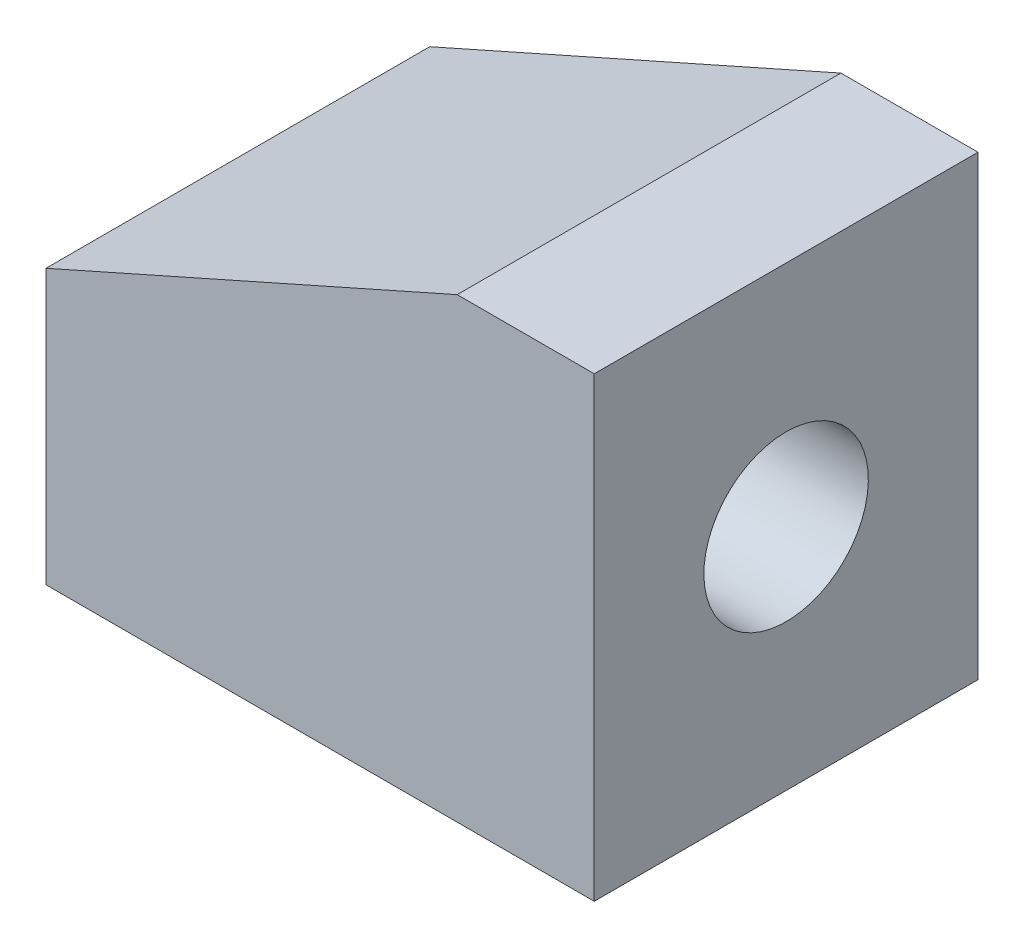
ISO-10303-21;
HEADER;
FILE_DESCRIPTION(('STEP AP214'),'2;1');
FILE_NAME('part.step','',(''),(''),'','','');
FILE_SCHEMA(('AUTOMOTIVE_DESIGN { 1 0 10303 214 1 1 1 1 }'));
ENDSEC;
DATA;
#1=APPLICATION_CONTEXT('core data for automotive mechanical design processes');
#2=APPLICATION_PROTOCOL_DEFINITION('international standard','automotive_design',2000,#1);
#3=PRODUCT_CONTEXT('',#1,'mechanical');
#4=PRODUCT('Part','Part','',(#3));
#5=PRODUCT_RELATED_PRODUCT_CATEGORY('part','',(#4));
#6=PRODUCT_DEFINITION_FORMATION('','',#4);
#7=PRODUCT_DEFINITION_CONTEXT('part definition',#1,'design');
#8=PRODUCT_DEFINITION('design','',#6,#7);
#9=PRODUCT_DEFINITION_SHAPE('','',#8);
#10=(LENGTH_UNIT() NAMED_UNIT(*) SI_UNIT(.MILLI.,.METRE.));
#11=(NAMED_UNIT(*) PLANE_ANGLE_UNIT() SI_UNIT($,.RADIAN.));
#12=(NAMED_UNIT(*) SI_UNIT($,.STERADIAN.) SOLID_ANGLE_UNIT());
#13=UNCERTAINTY_MEASURE_WITH_UNIT(LENGTH_MEASURE(1.E-05),#10,'distance_accuracy_value','');
#14=(GEOMETRIC_REPRESENTATION_CONTEXT(3) GLOBAL_UNCERTAINTY_ASSIGNED_CONTEXT((#13)) GLOBAL_UNIT_ASSIGNED_CONTEXT((#10,
#11,#12)) REPRESENTATION_CONTEXT('',''));
#15=CARTESIAN_POINT('',(0.,0.,0.));
#16=DIRECTION('',(0.,0.,1.));
#17=DIRECTION('',(1.,0.,0.));
#18=AXIS2_PLACEMENT_3D('',#15,#16,#17);
#19=CARTESIAN_POINT('',(-30.,0.,21.));
#20=DIRECTION('',(1.,0.,0.));
#21=DIRECTION('',(0.,0.,-1.));
#22=AXIS2_PLACEMENT_3D('',#19,#20,#21);
#23=PLANE('',#22);
#24=DIRECTION('',(0.,-1.,0.));
#25=VECTOR('',#24,1.);
#26=CARTESIAN_POINT('',(-30.,0.,-21.));
#27=LINE('',#26,#25);
#28=CARTESIAN_POINT('',(-30.,30.,-21.));
#29=VERTEX_POINT('',#28);
#30=CARTESIAN_POINT('',(-30.,0.,-21.));
#31=VERTEX_POINT('',#30);
#32=EDGE_CURVE('E117',#29,#31,#27,.T.);
#33=ORIENTED_EDGE('',*,*,#32,.T.);
#34=DIRECTION('',(0.,0.,-1.));
#35=VECTOR('',#34,1.);
#36=CARTESIAN_POINT('',(-30.,0.,21.));
#37=LINE('',#36,#35);
#38=CARTESIAN_POINT('',(-30.,0.,21.));
#39=VERTEX_POINT('',#38);
#40=EDGE_CURVE('E11',#39,#31,#37,.T.);
#41=ORIENTED_EDGE('',*,*,#40,.F.);
#42=DIRECTION('',(0.,-1.,0.));
#43=VECTOR('',#42,1.);
#44=CARTESIAN_POINT('',(-30.,0.,21.));
#45=LINE('',#44,#43);
#46=CARTESIAN_POINT('',(-30.,30.,21.));
#47=VERTEX_POINT('',#46);
#48=EDGE_CURVE('E127',#47,#39,#45,.T.);
#49=ORIENTED_EDGE('',*,*,#48,.F.);
#50=DIRECTION('',(0.,0.,-1.));
#51=VECTOR('',#50,1.);
#52=CARTESIAN_POINT('',(-30.,30.,21.));
#53=LINE('',#52,#51);
#54=EDGE_CURVE('E114',#47,#29,#53,.T.);
#55=ORIENTED_EDGE('',*,*,#54,.T.);
#56=EDGE_LOOP('',(#33,#41,#49,#55));
#57=FACE_BOUND('',#56,.T.);
#58=ADVANCED_FACE('F43',(#57),#23,.F.);
#59=CARTESIAN_POINT('',(30.,0.,21.));
#60=DIRECTION('',(0.,1.,0.));
#61=DIRECTION('',(0.,0.,1.));
#62=AXIS2_PLACEMENT_3D('',#59,#60,#61);
#63=PLANE('',#62);
#64=DIRECTION('',(1.,0.,0.));
#65=VECTOR('',#64,1.);
#66=CARTESIAN_POINT('',(30.,0.,-21.));
#67=LINE('',#66,#65);
#68=CARTESIAN_POINT('',(30.,0.,-21.));
#69=VERTEX_POINT('',#68);
#70=EDGE_CURVE('E120',#31,#69,#67,.T.);
#71=ORIENTED_EDGE('',*,*,#70,.T.);
#72=DIRECTION('',(0.,0.,-1.));
#73=VECTOR('',#72,1.);
#74=CARTESIAN_POINT('',(30.,0.,21.));
#75=LINE('',#74,#73);
#76=CARTESIAN_POINT('',(30.,0.,21.));
#77=VERTEX_POINT('',#76);
#78=EDGE_CURVE('E51',#77,#69,#75,.T.);
#79=ORIENTED_EDGE('',*,*,#78,.F.);
#80=DIRECTION('',(1.,0.,0.));
#81=VECTOR('',#80,1.);
#82=CARTESIAN_POINT('',(30.,0.,21.));
#83=LINE('',#82,#81);
#84=EDGE_CURVE('E91',#39,#77,#83,.T.);
#85=ORIENTED_EDGE('',*,*,#84,.F.);
#86=ORIENTED_EDGE('',*,*,#40,.T.);
#87=EDGE_LOOP('',(#71,#79,#85,#86));
#88=FACE_BOUND('',#87,.T.);
#89=ADVANCED_FACE('F144',(#88),#63,.F.);
#90=CARTESIAN_POINT('',(30.,50.,21.));
#91=DIRECTION('',(-1.,0.,0.));
#92=DIRECTION('',(0.,-1.,0.));
#93=AXIS2_PLACEMENT_3D('',#90,#91,#92);
#94=PLANE('',#93);
#95=CARTESIAN_POINT('',(30.,25.,0.));
#96=DIRECTION('',(1.,0.,0.));
#97=DIRECTION('',(0.,1.,0.));
#98=AXIS2_PLACEMENT_3D('',#95,#96,#97);
#99=CIRCLE('',#98,9.);
#100=CARTESIAN_POINT('',(30.,34.,0.));
#101=VERTEX_POINT('',#100);
#102=EDGE_CURVE('E159',#101,#101,#99,.T.);
#103=ORIENTED_EDGE('',*,*,#102,.F.);
#104=EDGE_LOOP('',(#103));
#105=FACE_BOUND('',#104,.T.);
#106=DIRECTION('',(0.,1.,0.));
#107=VECTOR('',#106,1.);
#108=CARTESIAN_POINT('',(30.,50.,-21.));
#109=LINE('',#108,#107);
#110=CARTESIAN_POINT('',(30.,50.,-21.));
#111=VERTEX_POINT('',#110);
#112=EDGE_CURVE('E107',#69,#111,#109,.T.);
#113=ORIENTED_EDGE('',*,*,#112,.T.);
#114=DIRECTION('',(0.,0.,-1.));
#115=VECTOR('',#114,1.);
#116=CARTESIAN_POINT('',(30.,50.,21.));
#117=LINE('',#116,#115);
#118=CARTESIAN_POINT('',(30.,50.,21.));
#119=VERTEX_POINT('',#118);
#120=EDGE_CURVE('E104',#119,#111,#117,.T.);
#121=ORIENTED_EDGE('',*,*,#120,.F.);
#122=DIRECTION('',(0.,1.,0.));
#123=VECTOR('',#122,1.);
#124=CARTESIAN_POINT('',(30.,50.,21.));
#125=LINE('',#124,#123);
#126=EDGE_CURVE('E100',#77,#119,#125,.T.);
#127=ORIENTED_EDGE('',*,*,#126,.F.);
#128=ORIENTED_EDGE('',*,*,#78,.T.);
#129=EDGE_LOOP('',(#113,#121,#127,#128));
#130=FACE_BOUND('',#129,.T.);
#131=ADVANCED_FACE('F106',(#105,#130),#94,.F.);
#132=CARTESIAN_POINT('',(15.,50.,21.));
#133=DIRECTION('',(0.,-1.,0.));
#134=DIRECTION('',(0.,0.,-1.));
#135=AXIS2_PLACEMENT_3D('',#132,#133,#134);
#136=PLANE('',#135);
#137=DIRECTION('',(-1.,0.,0.));
#138=VECTOR('',#137,1.);
#139=CARTESIAN_POINT('',(15.,50.,-21.));
#140=LINE('',#139,#138);
#141=CARTESIAN_POINT('',(15.,50.,-21.));
#142=VERTEX_POINT('',#141);
#143=EDGE_CURVE('E78',#111,#142,#140,.T.);
#144=ORIENTED_EDGE('',*,*,#143,.T.);
#145=DIRECTION('',(0.,0.,-1.));
#146=VECTOR('',#145,1.);
#147=CARTESIAN_POINT('',(15.,50.,21.));
#148=LINE('',#147,#146);
#149=CARTESIAN_POINT('',(15.,50.,21.));
#150=VERTEX_POINT('',#149);
#151=EDGE_CURVE('E108',#150,#142,#148,.T.);
#152=ORIENTED_EDGE('',*,*,#151,.F.);
#153=DIRECTION('',(-1.,0.,0.));
#154=VECTOR('',#153,1.);
#155=CARTESIAN_POINT('',(15.,50.,21.));
#156=LINE('',#155,#154);
#157=EDGE_CURVE('E101',#119,#150,#156,.T.);
#158=ORIENTED_EDGE('',*,*,#157,.F.);
#159=ORIENTED_EDGE('',*,*,#120,.T.);
#160=EDGE_LOOP('',(#144,#152,#158,#159));
#161=FACE_BOUND('',#160,.T.);
#162=ADVANCED_FACE('F112',(#161),#136,.F.);
#163=CARTESIAN_POINT('',(-30.,30.,21.));
#164=DIRECTION('',(0.406138466053448,-0.913811548620257,0.));
#165=DIRECTION('',(0.913811548620257,0.406138466053448,0.));
#166=AXIS2_PLACEMENT_3D('',#163,#164,#165);
#167=PLANE('',#166);
#168=DIRECTION('',(-0.913811548620257,-0.406138466053448,0.));
#169=VECTOR('',#168,1.);
#170=CARTESIAN_POINT('',(-30.,30.,-21.));
#171=LINE('',#170,#169);
#172=EDGE_CURVE('E84',#142,#29,#171,.T.);
#173=ORIENTED_EDGE('',*,*,#172,.T.);
#174=ORIENTED_EDGE('',*,*,#54,.F.);
#175=DIRECTION('',(-0.913811548620257,-0.406138466053448,0.));
#176=VECTOR('',#175,1.);
#177=CARTESIAN_POINT('',(-30.,30.,21.));
#178=LINE('',#177,#176);
#179=EDGE_CURVE('E56',#150,#47,#178,.T.);
#180=ORIENTED_EDGE('',*,*,#179,.F.);
#181=ORIENTED_EDGE('',*,*,#151,.T.);
#182=EDGE_LOOP('',(#173,#174,#180,#181));
#183=FACE_BOUND('',#182,.T.);
#184=ADVANCED_FACE('F133',(#183),#167,.F.);
#185=CARTESIAN_POINT('',(0.,0.,21.));
#186=DIRECTION('',(0.,0.,-1.));
#187=DIRECTION('',(-1.,0.,0.));
#188=AXIS2_PLACEMENT_3D('',#185,#186,#187);
#189=PLANE('',#188);
#190=ORIENTED_EDGE('',*,*,#48,.T.);
#191=ORIENTED_EDGE('',*,*,#84,.T.);
#192=ORIENTED_EDGE('',*,*,#126,.T.);
#193=ORIENTED_EDGE('',*,*,#157,.T.);
#194=ORIENTED_EDGE('',*,*,#179,.T.);
#195=EDGE_LOOP('',(#190,#191,#192,#193,#194));
#196=FACE_BOUND('',#195,.T.);
#197=ADVANCED_FACE('F97',(#196),#189,.F.);
#198=CARTESIAN_POINT('',(0.,0.,-21.));
#199=DIRECTION('',(0.,0.,-1.));
#200=DIRECTION('',(-1.,0.,0.));
#201=AXIS2_PLACEMENT_3D('',#198,#199,#200);
#202=PLANE('',#201);
#203=ORIENTED_EDGE('',*,*,#32,.F.);
#204=ORIENTED_EDGE('',*,*,#172,.F.);
#205=ORIENTED_EDGE('',*,*,#143,.F.);
#206=ORIENTED_EDGE('',*,*,#112,.F.);
#207=ORIENTED_EDGE('',*,*,#70,.F.);
#208=EDGE_LOOP('',(#203,#204,#205,#206,#207));
#209=FACE_BOUND('',#208,.T.);
#210=ADVANCED_FACE('F128',(#209),#202,.T.);
#211=CARTESIAN_POINT('',(-10.,25.,0.));
#212=DIRECTION('',(1.,0.,0.));
#213=DIRECTION('',(0.,1.,0.));
#214=AXIS2_PLACEMENT_3D('',#211,#212,#213);
#215=CYLINDRICAL_SURFACE('',#214,9.);
#216=CARTESIAN_POINT('',(-10.,25.,0.));
#217=DIRECTION('',(1.,0.,0.));
#218=DIRECTION('',(0.,1.,0.));
#219=AXIS2_PLACEMENT_3D('',#216,#217,#218);
#220=CIRCLE('',#219,9.);
#221=CARTESIAN_POINT('',(-10.,34.,0.));
#222=VERTEX_POINT('',#221);
#223=EDGE_CURVE('E123',#222,#222,#220,.T.);
#224=ORIENTED_EDGE('',*,*,#223,.F.);
#225=EDGE_LOOP('',(#224));
#226=FACE_BOUND('',#225,.T.);
#227=ORIENTED_EDGE('',*,*,#102,.T.);
#228=EDGE_LOOP('',(#227));
#229=FACE_BOUND('',#228,.T.);
#230=ADVANCED_FACE('F168',(#226,#229),#215,.F.);
#231=CARTESIAN_POINT('',(-10.,25.,0.));
#232=DIRECTION('',(1.,0.,0.));
#233=DIRECTION('',(0.,1.,0.));
#234=AXIS2_PLACEMENT_3D('',#231,#232,#233);
#235=PLANE('',#234);
#236=ORIENTED_EDGE('',*,*,#223,.T.);
#237=EDGE_LOOP('',(#236));
#238=FACE_BOUND('',#237,.T.);
#239=ADVANCED_FACE('F169',(#238),#235,.T.);
#240=CLOSED_SHELL('',(#58,#89,#131,#162,#184,#197,#210,#230,#239));
#241=MANIFOLD_SOLID_BREP('B2',#240);
#242=ADVANCED_BREP_SHAPE_REPRESENTATION('',(#18,#241),#14);
#243=SHAPE_DEFINITION_REPRESENTATION(#9,#242);
ENDSEC;
END-ISO-10303-21;
